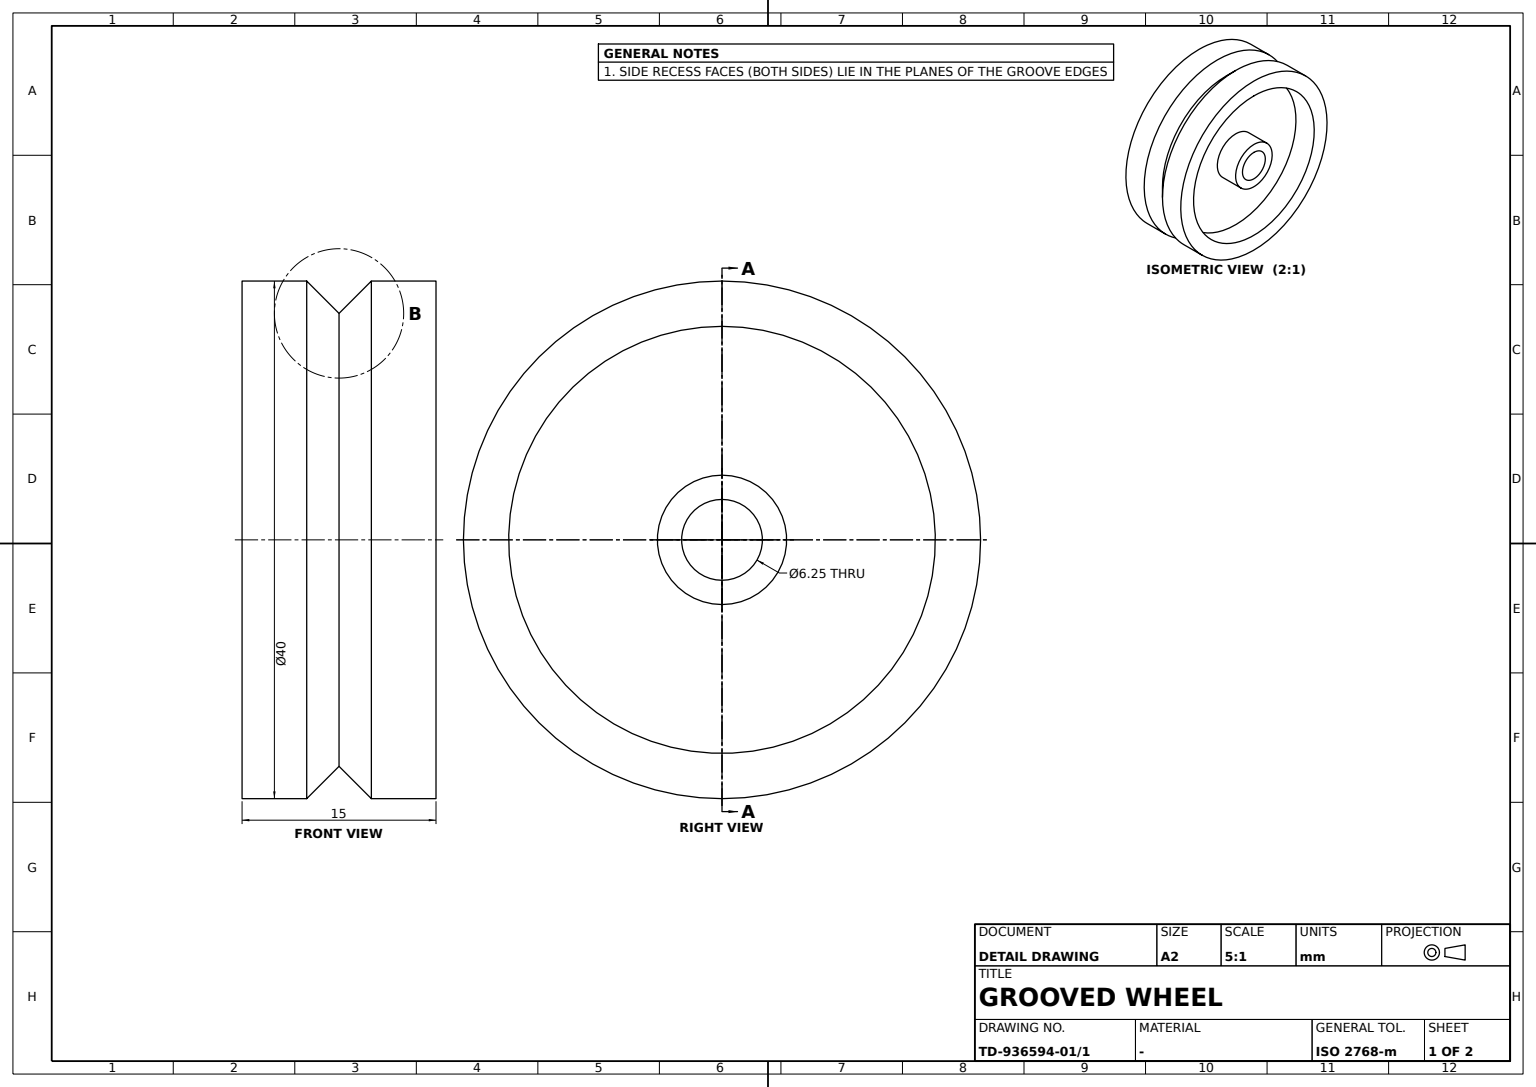
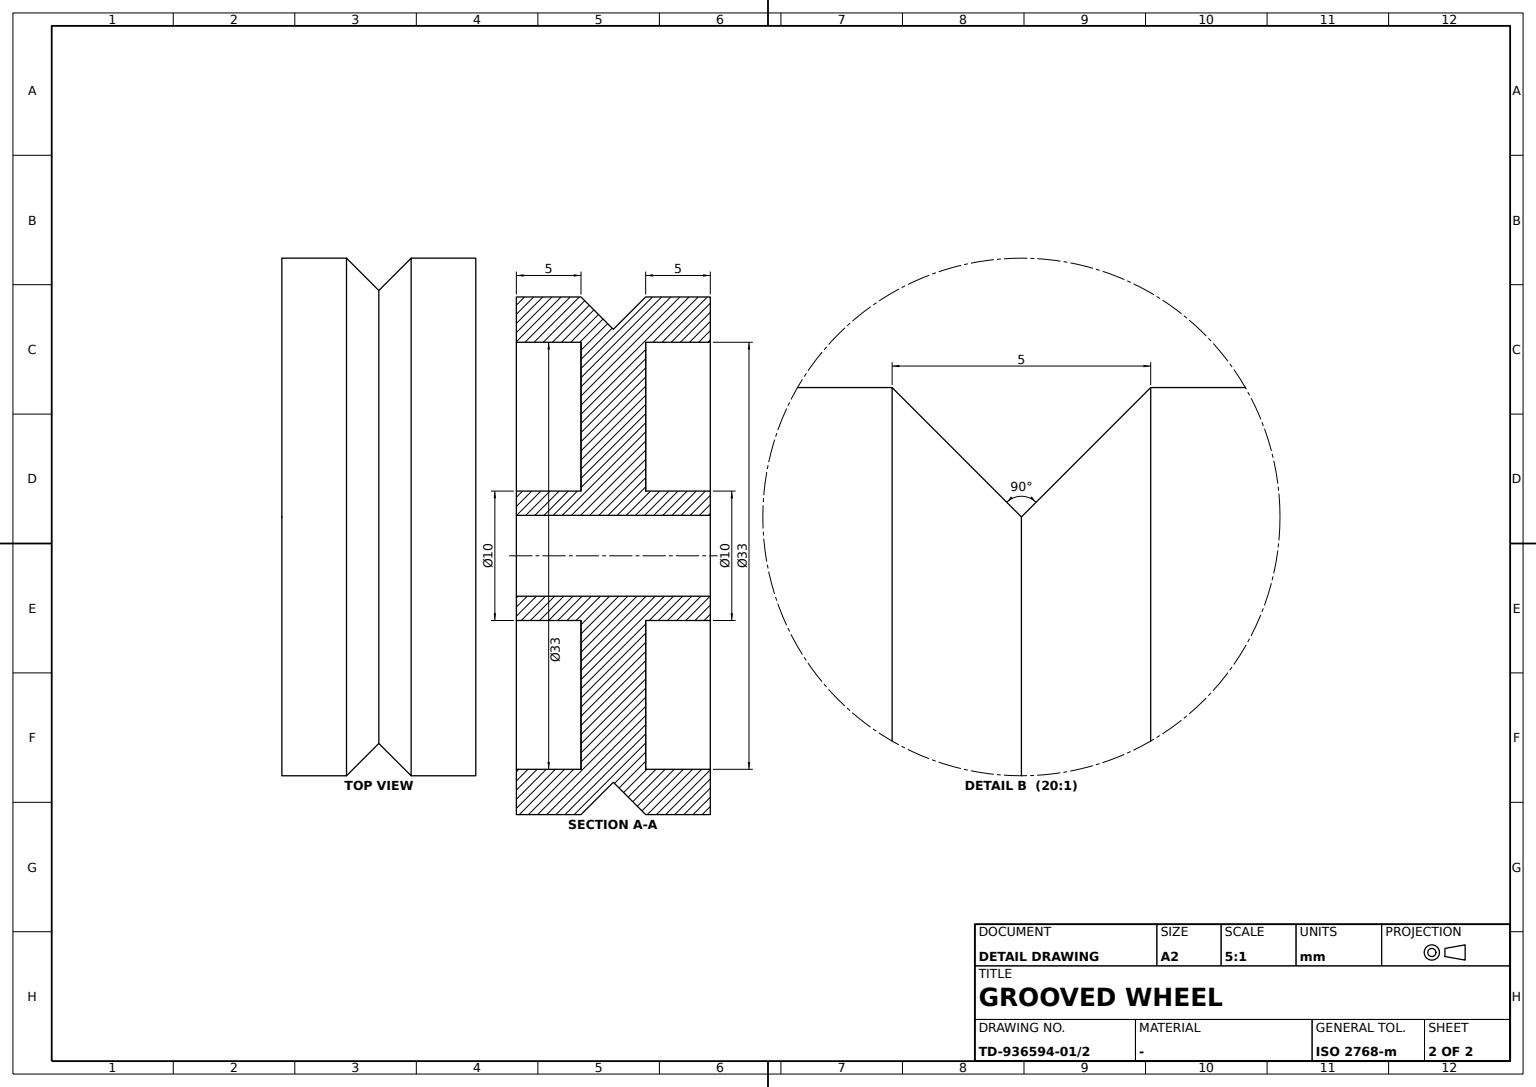
CATIA V5 part; units mm, degrees
sketch "Sketch1" plane through (0, 0, 0) normal (1, 0, 0) x (0, 1, 0)
  line L0 (0, 0) -> (7.5, 0)
  point P0 (7.5, 0)
  line L1 (7.5, 0) -> (7.5, 5)
  point P1 (7.5, 5)
  line L2 (7.5, 5) -> (2.5, 5)
  point P2 (2.5, 5)
  line L3 (2.5, 5) -> (2.5, 16.5)
  point P3 (2.5, 16.5)
  line L4 (2.5, 16.5) -> (7.5, 16.5)
  point P4 (7.5, 16.5)
  line L5 (7.5, 16.5) -> (7.5, 20)
  point P5 (7.5, 20)
  line L6 (7.5, 20) -> (2.5, 20)
  point P6 (2.5, 20)
  line L7 (2.5, 20) -> (0, 17.5)
  point P7 (-1.0355, 16.4645)
  point P8 (-2.5, 20)
  point P9 (-7.5, 20)
  line L8 (-7.5, 20) -> (-2.5, 20)
  point P10 (-7.5, 16.5)
  line L9 (-7.5, 16.5) -> (-7.5, 20)
  point P11 (-2.5, 16.5)
  line L10 (-2.5, 16.5) -> (-7.5, 16.5)
  line L11 (-2.5, 20) -> (0, 17.5)
  point P12 (-2.5, 5)
  line L12 (-2.5, 5) -> (-2.5, 16.5)
  point P13 (-7.5, 5)
  line L13 (-7.5, 5) -> (-2.5, 5)
  point P14 (-7.5, 0)
  line L14 (-7.5, 0) -> (-7.5, 5)
  point P15 (0, 0)
  line L15 (0, 0) -> (-7.5, 0)
  dimension "length L0" = 7.5
  dimension "distance L3 y axis" = 2.5
  dimension "distance L2 x axis" = 5
  dimension "distance L4 x axis" = 16.5
  dimension "distance L6 x axis" = 20
  dimension "angle L7 L11" = 90
  dimension "distance P6 P7" = 5
  constraint horizontal L0 x-axis
  constraint horizontal L2 x-axis
  constraint horizontal L4 x-axis
  constraint horizontal L6 x-axis
  constraint vertical L1 y-axis
  constraint vertical L3 y-axis
  constraint vertical L5 y-axis
  constraint coincidence P4 L1
  constraint coincidence P6 L3
  constraint coincidence origin P15
  constraint symmetry P6 P8 y-axis
  constraint symmetry P5 P9 y-axis
  constraint symmetry L6 L8 y-axis
  constraint symmetry P4 P10 y-axis
  constraint symmetry L5 L9 y-axis
  constraint symmetry P3 P11 y-axis
  constraint symmetry L4 L10 y-axis
  constraint symmetry L7 L11 y-axis
  constraint symmetry P2 P12 y-axis
  constraint symmetry L3 L12 y-axis
  constraint symmetry P1 P13 y-axis
  constraint symmetry L2 L13 y-axis
  constraint symmetry P0 P14 y-axis
  constraint symmetry L1 L14 y-axis
  constraint symmetry origin P15 y-axis
  constraint symmetry L0 L15 y-axis
revolve "Shaft1" add sketch "Sketch1" angle 360 about axis through (0, 0, 0) along (0, 1, 0)
sketch "Sketch2" plane through (0, 7.5, 0) normal (0, 1, 0) x (-1, 0, 0)
  circle A0 centre (0, 0) radius 3.125
  dimension "radius A0" = 3.125
extrude "Pocket1" cut sketch "Sketch2" against normal up to next
